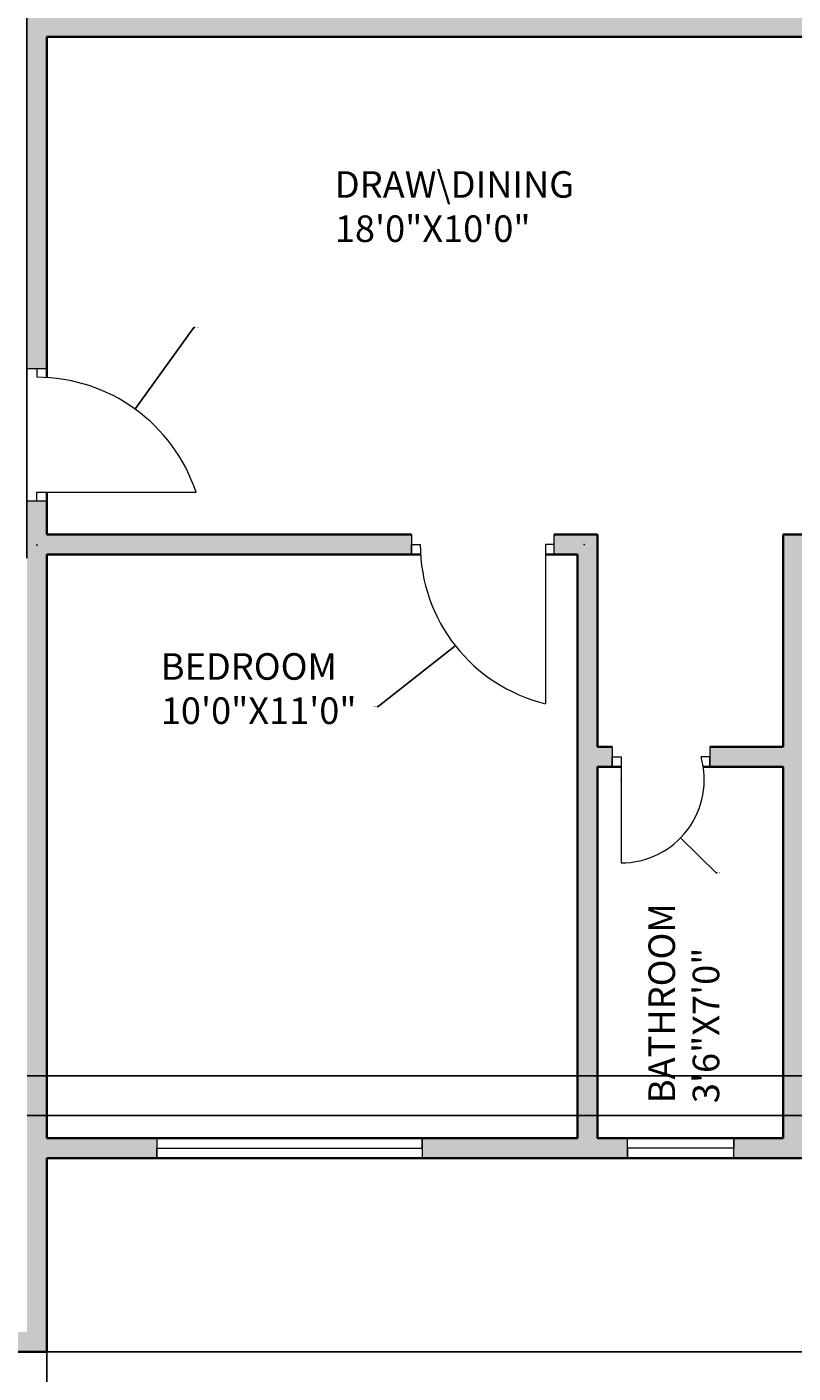
# Model space of a CAD drawing. Units: inches. Extents: x 2314 to 3223, y 1382 to 2735.
# Tile 4 of 14: x 2818 to 2992, y 1560 to 1864. Entities that reach past the tile are written whole.
import ezdxf

# ---------------------------------------------------------------- set-up
doc = ezdxf.new("R2010")
doc.units = ezdxf.units.IN
for name, color, linetype, lineweight in [('A-ANNO-DIMS', 2, 'Continuous', 18), ('A-AREA-IDEN', 7, 'Continuous', 18), ('A-DOOR', 3, 'Continuous', 18), ('A-GLAZ', 4, 'Continuous', 18), ('A-WALL', 7, 'Continuous', 35)]:
    doc.layers.add(name, color=color, linetype=linetype, lineweight=lineweight)
doc.layers.add('A-WALL-PATT', color=251, linetype='Continuous', lineweight=13, true_color=0x636466)
doc.styles.get("Standard").update_dxf_attribs({"font": 'arial.ttf'})
doc.dimstyles.get("Standard").update_dxf_attribs({"dimtxt": 0.18, "dimasz": 0.18, "dimexe": 0.18, "dimexo": 0.0625, "dimgap": 0.09, "dimtad": 0, "dimtih": 1, "dimtoh": 1, "dimdec": 4, "dimzin": 0, "dimdsep": 46, "dimtxsty": 'Standard', "dimcen": 0.09, "dimadec": 0, "dimazin": 0, "dimtfac": 1, "dimtdec": 4, "dimtofl": 0, "dimtmove": 0, "dimatfit": 3, "dimfxl": 1, "dimtolj": 1, "dimtzin": 0, "dimarcsym": 0})

# ---------------------------------------------------------------- blocks, each defined once
blk = doc.blocks.new('WIN-PLAN-24')
for p, q in [((0, 24), (4.5, 24)), ((4.5, 24), (2.25, 24)), ((2.25, 24), (2.25, 0)), ((2.25, 0), (0, 0)), ((0, 0), (4.5, 0))]:
    blk.add_line(p, q)
blk = doc.blocks.new('WIN-PLAN-60')
for p, q in [((0, 4.5), (0, 0)), ((60, 2.25), (60, 4.5)), ((60, 4.5), (60, 0)), ((0, 0), (0, 2.25)), ((0, 2.25), (60, 2.25))]:
    blk.add_line(p, q)
blk = doc.blocks.new('*D29')
at = {"layer": 'A-ANNO-DIMS', "color": 0, "lineweight": -2, "transparency": 16777216}
for p, q in [((2410.39, 1608.32), (2410.39, 1434.13)), ((3125.89, 1608.32), (3125.89, 1434.13)), ((2410.57, 1434.31), (2767.75, 1434.31)), ((3125.71, 1434.31), (2768.54, 1434.31))]:
    blk.add_line(p, q, dxfattribs=at)
at = {"layer": 'A-ANNO-DIMS', "color": 0, "transparency": 16777216}
for points in [[(2410.57, 1434.34), (2410.57, 1434.28), (2410.39, 1434.31)], [(3125.71, 1434.34), (3125.71, 1434.28), (3125.89, 1434.31)]]:
    blk.add_solid(points, dxfattribs=at)
at = {"layer": 'Defpoints', "color": 0, "transparency": 16777216}
for p in [(2410.39, 1608.38), (3125.89, 1608.38), (3125.89, 1434.31)]:
    blk.add_point(p, dxfattribs=at)
at = {"layer": 'A-ANNO-DIMS', "color": 0, "transparency": 16777216, "insert": (2768.14, 1434.31), "char_height": 0.18, "attachment_point": 5}
blk.add_mtext('\\A1;715.5', dxfattribs=at)
blk = doc.blocks.new('*D30')
at = {"layer": 'A-ANNO-DIMS', "color": 0, "lineweight": -2, "transparency": 16777216}
for p, q in [((3125.96, 2381.78), (3172.77, 2381.78)), ((3172.59, 2381.6), (3172.59, 1973.38)), ((3172.59, 1564.8), (3172.59, 1973.02)), ((2822.96, 1564.62), (3172.77, 1564.62))]:
    blk.add_line(p, q, dxfattribs=at)
at = {"layer": 'A-ANNO-DIMS', "color": 0, "transparency": 16777216}
for points in [[(3172.56, 2381.6), (3172.62, 2381.6), (3172.59, 2381.78)], [(3172.56, 1564.8), (3172.62, 1564.8), (3172.59, 1564.62)]]:
    blk.add_solid(points, dxfattribs=at)
at = {"layer": 'Defpoints', "color": 0, "transparency": 16777216}
for p in [(3125.89, 2381.78), (2822.89, 1564.62), (3172.59, 1564.62)]:
    blk.add_point(p, dxfattribs=at)
at = {"layer": 'A-ANNO-DIMS', "color": 0, "transparency": 16777216, "insert": (3172.59, 1973.2), "char_height": 0.18, "attachment_point": 5}
blk.add_mtext('\\A1;817.2', dxfattribs=at)
blk = doc.blocks.new('*D37')
at = {"layer": 'A-ANNO-DIMS', "color": 0, "lineweight": -2, "transparency": 16777216}
for p, q in [((2717.89, 1564.56), (2717.89, 1434.13)), ((2822.89, 1564.56), (2822.89, 1434.13)), ((2718.07, 1434.31), (2770.11, 1434.31)), ((2822.71, 1434.31), (2770.67, 1434.31))]:
    blk.add_line(p, q, dxfattribs=at)
at = {"layer": 'A-ANNO-DIMS', "color": 0, "transparency": 16777216}
for points in [[(2718.07, 1434.34), (2718.07, 1434.28), (2717.89, 1434.31)], [(2822.71, 1434.34), (2822.71, 1434.28), (2822.89, 1434.31)]]:
    blk.add_solid(points, dxfattribs=at)
at = {"layer": 'Defpoints', "color": 0, "transparency": 16777216}
for p in [(2717.89, 1564.62), (2822.89, 1564.62), (2822.89, 1434.31)]:
    blk.add_point(p, dxfattribs=at)
at = {"layer": 'A-ANNO-DIMS', "color": 0, "transparency": 16777216, "insert": (2770.39, 1434.31), "char_height": 0.18, "attachment_point": 5}
blk.add_mtext('\\A1;105', dxfattribs=at)
blk = doc.blocks.new('*D38')
at = {"layer": 'A-ANNO-DIMS', "color": 0, "lineweight": -2, "transparency": 16777216}
for p, q in [((2818.46, 1627), (3172.77, 1627)), ((3172.59, 1626.82), (3172.59, 1622.68)), ((3172.59, 1618.18), (3172.59, 1622.32)), ((2818.46, 1618), (3172.77, 1618))]:
    blk.add_line(p, q, dxfattribs=at)
at = {"layer": 'A-ANNO-DIMS', "color": 0, "transparency": 16777216}
for points in [[(3172.56, 1626.82), (3172.62, 1626.82), (3172.59, 1627)], [(3172.56, 1618.18), (3172.62, 1618.18), (3172.59, 1618)]]:
    blk.add_solid(points, dxfattribs=at)
at = {"layer": 'Defpoints', "color": 0, "transparency": 16777216}
for p in [(2818.39, 1627), (3172.59, 1627), (2818.39, 1618)]:
    blk.add_point(p, dxfattribs=at)
at = {"layer": 'A-ANNO-DIMS', "color": 0, "transparency": 16777216, "insert": (3172.59, 1622.5), "char_height": 0.18, "attachment_point": 5}
blk.add_mtext('\\A1;9', dxfattribs=at)
blk = doc.blocks.new('*D39')
at = {"layer": 'A-ANNO-DIMS', "color": 0, "lineweight": -2, "transparency": 16777216}
for p, q in [((2770.39, 1744.06), (2770.39, 2428.66)), ((2818.39, 1744.06), (2818.39, 2428.66)), ((2770.57, 2428.48), (2794.17, 2428.48)), ((2818.21, 2428.48), (2794.62, 2428.48))]:
    blk.add_line(p, q, dxfattribs=at)
at = {"layer": 'A-ANNO-DIMS', "color": 0, "transparency": 16777216}
for points in [[(2770.57, 2428.51), (2770.57, 2428.45), (2770.39, 2428.48)], [(2818.21, 2428.51), (2818.21, 2428.45), (2818.39, 2428.48)]]:
    blk.add_solid(points, dxfattribs=at)
at = {"layer": 'Defpoints', "color": 0, "transparency": 16777216}
for p in [(2818.39, 2428.48), (2770.39, 1744), (2818.39, 1744)]:
    blk.add_point(p, dxfattribs=at)
at = {"layer": 'A-ANNO-DIMS', "color": 0, "transparency": 16777216, "insert": (2794.39, 2428.48), "char_height": 0.18, "attachment_point": 5}
blk.add_mtext('\\A1;48', dxfattribs=at)
blk = doc.blocks.new('*D60')
at = {"layer": 'A-ANNO-DIMS', "color": 0, "lineweight": -2, "transparency": 16777216}
for p, q in [((2856.17, 1796.19), (2842.95, 1777.89)), ((2856.35, 1796.19), (2856.17, 1796.19)), ((2820.55, 1747), (2820.73, 1747)), ((2820.64, 1746.91), (2820.64, 1747.09))]:
    blk.add_line(p, q, dxfattribs=at)
at = {"layer": 'A-ANNO-DIMS', "color": 0, "transparency": 16777216}
blk.add_solid([(2842.93, 1777.91), (2842.98, 1777.87), (2842.85, 1777.74)], dxfattribs=at)
at = {"layer": 'Defpoints', "color": 0, "transparency": 16777216}
for p in [(2842.85, 1777.74), (2820.64, 1747)]:
    blk.add_point(p, dxfattribs=at)
at = {"layer": 'A-ANNO-DIMS', "color": 0, "transparency": 16777216, "insert": (2856.83, 1796.19), "char_height": 0.18, "attachment_point": 5}
blk.add_mtext('\\A1;R37.92', dxfattribs=at)
blk = doc.blocks.new('*D62')
at = {"layer": 'A-ANNO-DIMS', "color": 0, "lineweight": -2, "transparency": 16777216}
for p, q in [((2944.31, 1747.13), (2944.49, 1747.13)), ((2944.4, 1747.04), (2944.4, 1747.22)), ((2897.8, 1710.5), (2915.13, 1724.13)), ((2897.62, 1710.5), (2897.8, 1710.5))]:
    blk.add_line(p, q, dxfattribs=at)
at = {"layer": 'A-ANNO-DIMS', "color": 0, "transparency": 16777216}
blk.add_solid([(2915.11, 1724.15), (2915.15, 1724.1), (2915.27, 1724.24)], dxfattribs=at)
at = {"layer": 'Defpoints', "color": 0, "transparency": 16777216}
for p in [(2944.4, 1747.13), (2915.27, 1724.24)]:
    blk.add_point(p, dxfattribs=at)
at = {"layer": 'A-ANNO-DIMS', "color": 0, "transparency": 16777216, "insert": (2897.14, 1710.5), "char_height": 0.18, "attachment_point": 5}
blk.add_mtext('\\A1;R37.05', dxfattribs=at)
blk = doc.blocks.new('*D94')
at = {"layer": 'A-ANNO-DIMS', "color": 0, "lineweight": -2, "transparency": 16777216}
for p, q in [((2952.67, 1693.93), (2952.85, 1693.93)), ((2952.76, 1693.84), (2952.76, 1694.02)), ((2974.26, 1672.9), (2966.32, 1680.66)), ((2974.44, 1672.9), (2974.26, 1672.9))]:
    blk.add_line(p, q, dxfattribs=at)
at = {"layer": 'A-ANNO-DIMS', "color": 0, "transparency": 16777216}
blk.add_solid([(2966.35, 1680.68), (2966.3, 1680.64), (2966.2, 1680.79)], dxfattribs=at)
at = {"layer": 'Defpoints', "color": 0, "transparency": 16777216}
for p in [(2952.76, 1693.93), (2966.2, 1680.79)]:
    blk.add_point(p, dxfattribs=at)
at = {"layer": 'A-ANNO-DIMS', "color": 0, "transparency": 16777216, "insert": (2974.85, 1672.9), "char_height": 0.18, "attachment_point": 5}
blk.add_mtext('\\A1;R18.8', dxfattribs=at)

msp = doc.modelspace()

# ---------------------------------------------------------------- hatches: boundary and pattern name
at = {"layer": 'A-WALL-PATT'}
h = msp.add_hatch(color=256, dxfattribs=at)
h.dxf.hatch_style = 1
h.paths.add_polyline_path([(2443.3302, 2379.5332), (2443.3302, 2381.7832), (2410.3927, 2381.7832), (2410.3927, 2336.7008), (2414.8927, 2336.7008), (2414.8927, 2377.2832), (2443.3302, 2377.2832)])
h.paths.add_polyline_path([(2561.3645, 2379.5332), (2561.3645, 2381.7832), (2503.3302, 2381.7832), (2503.3302, 2377.2832), (2546.8927, 2377.2832), (2546.8927, 2245.2832), (2541.8787, 2245.2832), (2541.8787, 2240.7832), (2551.3927, 2240.7832), (2551.3927, 2377.2832), (2561.3645, 2377.2832)])
h.paths.add_polyline_path([(2656.0607, 2381.7832), (2597.3645, 2381.7832), (2597.3645, 2377.2832), (2617.3927, 2377.2832), (2617.3927, 2257.2832), (2584.2532, 2257.2832), (2584.2532, 2252.7832), (2625.8528, 2252.7832), (2625.8528, 2255.0332), (2625.8528, 2257.2832), (2621.8927, 2257.2832), (2621.8927, 2377.2832), (2656.0607, 2377.2832), (2656.0607, 2379.5332)])
h.paths.add_polyline_path([(2807.3418, 2381.7832), (2716.0607, 2381.7832), (2716.0607, 2377.2832), (2765.8927, 2377.2832), (2765.8927, 2257.2832), (2661.6935, 2257.2832), (2661.6935, 2252.7832), (2765.8927, 2252.7832), (2765.8927, 2146.2832), (2760.9259, 2146.2832), (2760.9259, 2141.8832), (2775.7119, 2141.8832), (2775.7119, 2146.2832), (2770.3927, 2146.2832), (2770.3927, 2252.7832), (2877.684, 2252.7832), (2877.684, 2255.0332), (2877.684, 2257.2832), (2770.3927, 2257.2832), (2770.3927, 2377.2832), (2807.3418, 2377.2832), (2807.3418, 2379.5332)])
h.paths.add_polyline_path([(2937.2118, 2381.7832), (2867.3418, 2381.7832), (2867.3418, 2377.2832), (2914.3927, 2377.2832), (2914.3927, 2257.2832), (2908.4124, 2257.2832), (2908.4124, 2252.7832), (2960.6432, 2252.7832), (2960.6432, 2255.0332), (2960.6432, 2257.2832), (2918.8927, 2257.2832), (2918.8927, 2377.2832), (2937.2118, 2377.2832)])
h.paths.add_polyline_path([(3022.1601, 2381.7832), (2973.2118, 2381.7832), (2973.2118, 2379.5332), (2973.2118, 2377.2832), (2984.8927, 2377.2832), (2984.8927, 2257.2832), (2980.0601, 2257.2832), (2980.0601, 2252.7832), (2984.8927, 2252.7832), (2984.8927, 2240.7832), (2995.668, 2240.7832), (2995.668, 2243.0332), (2995.668, 2245.2832), (2989.3927, 2245.2832), (2989.3927, 2377.2832), (3022.1601, 2377.2832), (3022.1601, 2379.5332)])
h.paths.add_polyline_path([(3125.8927, 2381.7832), (3082.1601, 2381.7832), (3082.1601, 2377.2832), (3121.3927, 2377.2832), (3121.3927, 2334.7388), (3125.8927, 2334.7388)])
h.paths.add_polyline_path([(3125.8927, 2274.7388), (3121.3927, 2274.7388), (3121.3927, 2245.2832), (3066.4832, 2245.2832), (3066.4832, 2240.7832), (3121.3927, 2240.7832), (3121.3927, 2232.1868), (3125.8927, 2232.1868)])
h.paths.add_polyline_path([(3125.8927, 2208.1868), (3121.3927, 2208.1868), (3121.3927, 2198.7832), (3037.3927, 2198.7832), (3037.3927, 2240.7832), (3041.2694, 2240.7832), (3041.2694, 2243.0332), (3041.2694, 2245.2832), (3026.8205, 2245.2832), (3026.8205, 2240.7832), (3032.8927, 2240.7832), (3032.8927, 2190.4022), (3037.3927, 2190.4022), (3037.3927, 2194.2832), (3121.3927, 2194.2832), (3121.3927, 2182.1835), (3125.8927, 2182.1835)])
h.paths.add_polyline_path([(3125.8927, 2158.1835), (3121.3927, 2158.1835), (3121.3927, 2146.2832), (3037.3927, 2146.2832), (3037.3927, 2169.3726), (3035.1427, 2169.3726), (3032.8927, 2169.3726), (3032.8927, 2146.2832), (2812.7301, 2146.2832), (2812.7301, 2144.0832), (2812.7301, 2141.8832), (2818.3927, 2141.8832), (2818.3927, 1970.1316), (2822.8927, 1970.1316), (2822.8927, 1978.8832), (2903.9846, 1978.8832), (2903.9846, 1981.1332), (2903.9846, 1983.3832), (2822.8927, 1983.3832), (2822.8927, 2115.3832), (2851.7162, 2115.3832), (2851.7162, 2117.6332), (2851.7162, 2119.8832), (2822.8927, 2119.8832), (2822.8927, 2141.8832), (3125.8927, 2141.8832)])
h.paths.add_polyline_path([(3125.8927, 2119.8832), (3081.193, 2119.8832), (3081.193, 2115.3832), (3121.3927, 2115.3832), (3121.3927, 2071.8188), (3125.8927, 2071.8188)], flags=17)
h.paths.add_polyline_path([(2989.3927, 2115.3832), (3021.193, 2115.3832), (3021.193, 2117.6332), (3021.193, 2119.8832), (2979.123, 2119.8832), (2979.123, 2115.3832), (2984.8927, 2115.3832), (2984.8927, 2019.3832), (2981.9225, 2019.3832), (2981.9225, 2014.8832), (2984.8927, 2014.8832), (2984.8927, 1983.3832), (2984.8927, 1978.8832), (2989.3927, 1978.8832), (2989.3927, 1983.3832)], flags=17)
h.paths.add_polyline_path([(2947.3927, 2115.3832), (2955.123, 2115.3832), (2955.123, 2117.6332), (2955.123, 2119.8832), (2911.7162, 2119.8832), (2911.7162, 2115.3832), (2942.8927, 2115.3832), (2942.8927, 1983.3832), (2936.7017, 1983.3832), (2936.7017, 1978.8832), (2947.3927, 1978.8832), (2947.3927, 1983.3832), (2947.3927, 2014.8832), (2960.7167, 2014.8832), (2960.7167, 2017.1332), (2960.7167, 2019.3832), (2947.3927, 2019.3832)], flags=17)
h.paths.add_polyline_path([(3037.3927, 1978.8832), (3041.8276, 1978.8832), (3041.8276, 1981.1332), (3041.8276, 1983.3832), (3025.477, 1983.3832), (3025.477, 1978.8832), (3032.8927, 1978.8832), (3032.8927, 1927.1259), (3035.1427, 1927.1259), (3037.3927, 1927.1259)])
h.paths.add_polyline_path([(3125.8927, 2011.8188), (3123.6427, 2011.8188), (3121.3927, 2011.8188), (3121.3927, 1983.3832), (3065, 1983.3832), (3065, 1978.8832), (3121.3927, 1978.8832), (3121.3927, 1970.5932), (3125.8927, 1970.5932)], flags=17)
h.paths.add_polyline_path([(2994.2341, 1983.3832), (2989.3927, 1983.3832), (2989.3927, 1978.8832), (2994.2341, 1978.8832), (2994.2341, 1981.1332)], flags=16)
h.paths.add_polyline_path([(3125.8927, 1946.5932), (3121.3927, 1946.5932), (3121.3927, 1936.8832), (3037.3927, 1936.8832), (3037.3927, 1932.3832), (3121.3927, 1932.3832), (3121.3927, 1919.825), (3125.8927, 1919.825)])
h.paths.add_polyline_path([(3125.8927, 1883.825), (3121.3927, 1883.825), (3121.3927, 1866.3832), (3037.3927, 1866.3832), (3037.3927, 1899.0954), (3035.1427, 1899.0954), (3032.8927, 1899.0954), (3032.8927, 1866.3832), (2822.8927, 1866.3832), (2822.8927, 1938.7212), (2820.6427, 1938.7212), (2818.3927, 1938.7212), (2818.3927, 1786.9239), (2822.8927, 1786.9239), (2822.8927, 1861.8832), (3032.8927, 1861.8832), (3032.8927, 1825.1023), (3037.3927, 1825.1023), (3037.3927, 1861.8832), (3121.3927, 1861.8832), (3121.3927, 1844.6765), (3125.8927, 1844.6765)])
h.paths.add_polyline_path([(3125.8927, 1808.6765), (3121.3927, 1808.6765), (3121.3927, 1795.8832), (3037.3927, 1795.8832), (3037.3927, 1799.4755), (3032.8927, 1799.4755), (3032.8927, 1749.3832), (3026.5034, 1749.3832), (3026.5034, 1744.8832), (3032.8927, 1744.8832), (3034.9255, 1744.8832), (3043.1326, 1744.8832), (3043.1326, 1747.1332), (3043.1326, 1749.3832), (3037.3927, 1749.3832), (3037.3927, 1791.3832), (3121.3927, 1791.3832), (3121.3927, 1783.3103), (3125.8927, 1783.3103)])
h.paths.add_polyline_path([(3125.8927, 1759.3103), (3121.3927, 1759.3103), (3121.3927, 1749.3832), (3065.1845, 1749.3832), (3065.1845, 1744.8832), (3121.3927, 1744.8832), (3121.3927, 1709.3573), (3125.8927, 1709.3573)])
h.paths.add_polyline_path([(3125.8927, 1649.3573), (3121.3927, 1649.3573), (3121.3927, 1612.8832), (3095.116, 1612.8832), (3095.116, 1608.3832), (3125.8927, 1608.3832)])
h.paths.add_polyline_path([(3035.116, 1612.8832), (2993.8927, 1612.8832), (2993.8927, 1744.8832), (2998.7409, 1744.8832), (2998.7409, 1749.3832), (2989.3927, 1749.3832), (2989.3927, 1744.8832), (2989.3927, 1701.3832), (2972.8226, 1701.3832), (2972.8226, 1696.8832), (2989.3927, 1696.8832), (2989.3927, 1612.8832), (2978.2225, 1612.8832), (2978.2225, 1608.3832), (3035.116, 1608.3832), (3035.116, 1610.6332)])
h.paths.add_polyline_path([(2947.3927, 1696.8832), (2950.7566, 1696.8832), (2950.7566, 1699.1332), (2950.7566, 1701.3832), (2947.3927, 1701.3832), (2947.3927, 1744.8832), (2947.3927, 1749.3832), (2937.649, 1749.3832), (2937.649, 1744.8832), (2942.8927, 1744.8832), (2942.8927, 1612.8832), (2907.783, 1612.8832), (2907.783, 1608.3832), (2954.2225, 1608.3832), (2954.2225, 1610.6332), (2954.2225, 1612.8832), (2947.3927, 1612.8832)])
h.paths.add_polyline_path([(2822.8927, 1744.8832), (2905.3491, 1744.8832), (2905.3491, 1747.1332), (2905.3491, 1749.3832), (2822.8927, 1749.3832), (2822.8927, 1756.9185), (2818.3927, 1756.9185), (2818.3927, 1612.8832), (2818.3927, 1569.1205), (2722.3927, 1569.1205), (2722.3927, 1612.8832), (2722.3927, 1756.9185), (2717.8927, 1756.9185), (2717.8927, 1750.0143), (2633.6297, 1750.0143), (2633.6437, 1745.2665), (2717.8927, 1745.5143), (2717.8927, 1612.8832), (2689.8467, 1612.8832), (2689.8467, 1608.3832), (2717.8927, 1608.3832), (2717.8927, 1564.6205), (2722.3927, 1564.6205), (2822.8927, 1564.6205), (2822.8927, 1569.1205), (2822.8927, 1608.3832), (2847.783, 1608.3832), (2847.783, 1610.6332), (2847.783, 1612.8832), (2822.8927, 1612.8832)])
h.paths.add_polyline_path([(2629.8467, 1612.8832), (2597.8927, 1612.8832), (2597.8927, 1744.8832), (2597.8927, 1745.1613), (2601.5887, 1745.1721), (2601.5816, 1747.5932), (2601.5745, 1750.0143), (2593.3927, 1750.0143), (2593.3927, 1744.8832), (2593.3927, 1713.3832), (2589.7588, 1713.3832), (2589.7588, 1708.8832), (2593.3927, 1708.8832), (2593.3927, 1612.8832), (2582.3793, 1612.8832), (2582.3793, 1608.3832), (2629.8467, 1608.3832), (2629.8467, 1610.6332)])
h.paths.add_polyline_path([(2551.3927, 1708.8832), (2567.6776, 1708.8832), (2567.6776, 1711.1332), (2567.6776, 1713.3832), (2551.3927, 1713.3832), (2551.3927, 1744.8832), (2551.3927, 1750.0143), (2543.5657, 1750.0143), (2543.5657, 1747.5079), (2543.5657, 1745.0014), (2546.8927, 1745.0112), (2546.8927, 1744.8832), (2546.8927, 1612.8832), (2502.9339, 1612.8832), (2502.9339, 1608.3832), (2558.3793, 1608.3832), (2558.3793, 1610.6332), (2558.3793, 1612.8832), (2551.3927, 1612.8832)])
h.paths.add_polyline_path([(2414.8927, 1656.2547), (2410.3927, 1656.2547), (2410.3927, 1608.3832), (2442.9339, 1608.3832), (2442.9339, 1610.6332), (2442.9339, 1612.8832), (2414.8927, 1612.8832)])
h.paths.add_polyline_path([(2414.8927, 1744.8832), (2468.8906, 1744.8832), (2468.8906, 1747.1332), (2468.8906, 1749.3832), (2414.8927, 1749.3832), (2414.8927, 1757.7622), (2410.3927, 1757.7622), (2410.3927, 1716.2547), (2414.8927, 1716.2547)])
h.paths.add_polyline_path([(2414.8927, 1791.3832), (2498.8927, 1791.3832), (2498.8927, 1749.3832), (2492.9799, 1749.3832), (2492.9799, 1744.8832), (2498.8927, 1744.8832), (2503.3927, 1744.8832), (2508.0135, 1744.8968), (2508.0059, 1747.4556), (2507.9984, 1750.0143), (2503.3927, 1750.0143), (2503.3927, 1802.6362), (2501.1427, 1802.6362), (2498.8927, 1802.6362), (2498.8927, 1795.8832), (2414.8927, 1795.8832), (2414.8927, 1808.0943), (2410.3927, 1808.0943), (2410.3927, 1781.7622), (2414.8927, 1781.7622)])
h.paths.add_polyline_path([(2722.3927, 1937.589), (2720.1427, 1937.589), (2717.8927, 1937.589), (2717.8927, 1866.3832), (2503.3927, 1866.3832), (2503.3927, 1896.3484), (2498.8927, 1896.3484), (2498.8927, 1866.3832), (2414.8927, 1866.3832), (2414.8927, 1882.1496), (2410.3927, 1882.1496), (2410.3927, 1844.0943), (2414.8927, 1844.0943), (2414.8927, 1861.8832), (2498.8927, 1861.8832), (2498.8927, 1831.4783), (2501.1427, 1831.4783), (2503.3927, 1831.4783), (2503.3927, 1861.8832), (2717.8927, 1861.8832), (2717.8927, 1786.9239), (2722.3927, 1786.9239)])
h.paths.add_polyline_path([(2414.8927, 1932.3832), (2498.8927, 1932.3832), (2498.8927, 1924.7883), (2503.3927, 1924.7883), (2503.3927, 1978.8832), (2505.8599, 1978.8832), (2505.8599, 1981.1332), (2505.8599, 1983.3832), (2493.3697, 1983.3832), (2493.3697, 1978.8832), (2498.8927, 1978.8832), (2498.8927, 1936.8832), (2414.8927, 1936.8832), (2414.8927, 1943.2834), (2410.3927, 1943.2834), (2410.3927, 1918.1496), (2414.8927, 1918.1496)])
h.paths.add_polyline_path([(2414.8927, 2020.3133), (2412.6427, 2020.3133), (2410.3927, 2020.3133), (2410.3927, 1967.2834), (2414.8927, 1967.2834), (2414.8927, 1978.8832), (2468.8513, 1978.8832), (2468.8513, 1981.1332), (2468.8513, 1983.3832), (2414.8927, 1983.3832)])
h.paths.add_polyline_path([(2414.8927, 2115.3832), (2453.004, 2115.3832), (2453.004, 2117.6332), (2453.004, 2119.8832), (2410.3927, 2119.8832), (2410.3927, 2080.3133), (2414.8927, 2080.3133)], flags=17)
h.paths.add_polyline_path([(2559.0969, 2117.6332), (2559.0969, 2119.8832), (2513.004, 2119.8832), (2513.004, 2115.3832), (2546.8927, 2115.3832), (2546.8927, 1983.3832), (2542.7531, 1983.3832), (2542.7531, 1978.8832), (2551.3927, 1978.8832), (2551.3927, 2014.8832), (2570.3098, 2014.8832), (2570.3098, 2017.1332), (2570.3098, 2019.3832), (2551.3927, 2019.3832), (2551.3927, 2115.3832), (2559.0969, 2115.3832)], flags=17)
h.paths.add_polyline_path([(2628.5073, 2117.6332), (2628.5073, 2119.8832), (2583.0969, 2119.8832), (2583.0969, 2115.3832), (2593.3927, 2115.3832), (2593.3927, 2019.3832), (2590.2108, 2019.3832), (2590.2108, 2014.8832), (2593.3927, 2014.8832), (2593.3927, 1978.8832), (2601.5907, 1978.8832), (2601.5907, 1981.1332), (2601.5907, 1983.3832), (2597.8927, 1983.3832), (2597.8927, 2115.3832), (2628.5073, 2115.3832)], flags=17)
h.paths.add_polyline_path([(2722.3927, 2141.8832), (2726.9871, 2141.8832), (2726.9871, 2144.2705), (2726.9871, 2146.2832), (2503.3927, 2146.2832), (2503.3927, 2168.2161), (2501.1427, 2168.2161), (2498.8927, 2168.2161), (2498.8927, 2146.2832), (2414.8927, 2146.2832), (2414.8927, 2156.5041), (2410.3927, 2156.5041), (2410.3927, 2141.8832), (2717.8927, 2141.8832), (2717.8927, 2119.8832), (2688.5073, 2119.8832), (2688.5073, 2115.3832), (2717.8927, 2115.3832), (2717.8927, 1983.3832), (2633.2454, 1983.3832), (2633.2454, 1978.8832), (2717.8927, 1978.8832), (2717.8927, 1970.1316), (2720.1427, 1970.1316), (2722.3927, 1970.1316)])
h.paths.add_polyline_path([(2557.3704, 1462.9278), (2940.0934, 1462.9278), (2940.0934, 1512.3848), (2557.3704, 1512.3848)], flags=9)
h.paths.add_polyline_path([(2846.2527, 1703.1384), (2892.8612, 1703.1384), (2892.8612, 1725.5272), (2846.2527, 1725.5272)], flags=25)
h.paths.add_polyline_path([(2885.6102, 1812.1147), (2946.1505, 1812.1147), (2946.1505, 1834.5035), (2885.6102, 1834.5035)], flags=25)
h.paths.add_polyline_path([(2885.6102, 1884.183), (2946.1505, 1884.183), (2946.1505, 1906.5718), (2885.6102, 1906.5718)], flags=25)
h.paths.add_polyline_path([(3066.365, 1705.5431), (3112.9735, 1705.5431), (3112.9735, 1727.9319), (3066.365, 1727.9319)], flags=9)
h.paths.add_polyline_path([(3061.8255, 1887.7513), (3101.6154, 1887.7513), (3101.6154, 1910.1401), (3061.8255, 1910.1401)], flags=25)
h.paths.add_polyline_path([(3063.3679, 1816.2121), (3103.1578, 1816.2121), (3103.1578, 1838.6009), (3063.3679, 1838.6009)], flags=25)
h.paths.add_polyline_path([(3053.3743, 1768.416), (3107.1329, 1768.416), (3107.1329, 1790.8048), (3053.3743, 1790.8048)], flags=25)
h.paths.add_polyline_path([(3061.6068, 1943.822), (3115.3653, 1943.822), (3115.3653, 1966.2109), (3061.6068, 1966.2109)], flags=9)
h.paths.add_polyline_path([(2745.0978, 1763.6604), (2797.9354, 1763.6604), (2797.9354, 1776.0247), (2745.0978, 1776.0247)], flags=9)
h.paths.add_polyline_path([(2574.2135, 1819.2586), (2634.7538, 1819.2586), (2634.7538, 1841.6474), (2574.2135, 1841.6474)], flags=25)
h.paths.add_polyline_path([(2574.2135, 1891.3269), (2634.7538, 1891.3269), (2634.7538, 1913.7157), (2574.2135, 1913.7157)], flags=25)
h.paths.add_polyline_path([(2638.4466, 1702.43), (2685.0551, 1702.43), (2685.0551, 1724.8188), (2638.4466, 1724.8188)], flags=25)
h.paths.add_polyline_path([(2435.9715, 1697.1215), (2482.5799, 1697.1215), (2482.5799, 1719.5103), (2435.9715, 1719.5103)], flags=9)
h.paths.add_polyline_path([(2431.2046, 1893.7833), (2470.9945, 1893.7833), (2470.9945, 1916.1721), (2431.2046, 1916.1721)], flags=25)
h.paths.add_polyline_path([(2439.8144, 1817.2116), (2479.6043, 1817.2116), (2479.6043, 1839.6004), (2439.8144, 1839.6004)], flags=25)
h.paths.add_polyline_path([(2441.2607, 1753.0942), (2495.0192, 1753.0942), (2495.0192, 1775.483), (2441.2607, 1775.483)], flags=25)
h.paths.add_polyline_path([(2421.216, 1945.3109), (2474.9746, 1945.3109), (2474.9746, 1967.6997), (2421.216, 1967.6997)], flags=25)
h.paths.add_polyline_path([(2585.4464, 1627.5703), (2585.4464, 1679), (2563.0576, 1679), (2563.0576, 1627.5703)], flags=9)
h.paths.add_polyline_path([(2978.3497, 1618.7039), (2978.3497, 1670.1337), (2955.9609, 1670.1337), (2955.9609, 1618.7039)], flags=9)
h.paths.add_polyline_path([(2975.9502, 2041.7828), (2975.9502, 2093.2125), (2953.5614, 2093.2125), (2953.5614, 2041.7828)], flags=25)
h.paths.add_polyline_path([(2835.6537, 1989.2068), (2882.2621, 1989.2068), (2882.2621, 2011.5956), (2835.6537, 2011.5956)], flags=25)
h.paths.add_polyline_path([(2649.3769, 1997.5659), (2695.9853, 1997.5659), (2695.9853, 2019.9547), (2649.3769, 2019.9547)], flags=25)
h.paths.add_polyline_path([(2579.9087, 2040.3429), (2579.9087, 2091.7726), (2557.5198, 2091.7726), (2557.5198, 2040.3429)], flags=25)
h.paths.add_polyline_path([(2783.2404, 1883.1956), (2783.2404, 2067.1369), (2764.694, 2067.1369), (2764.694, 1883.1956)], flags=9)
h.paths.add_polyline_path([(3055.8435, 1993.5571), (3102.4519, 1993.5571), (3102.4519, 2015.9459), (3055.8435, 2015.9459)], flags=25)
h.paths.add_polyline_path([(2423.6009, 1984.6082), (2470.2094, 1984.6082), (2470.2094, 2006.997), (2423.6009, 2006.997)], flags=25)
h.paths.add_polyline_path([(2973.4115, 2123.1668), (3013.1319, 2123.1668), (3013.1319, 2135.531), (2973.4115, 2135.531)], flags=25)
h.paths.add_polyline_path([(2534.3846, 2124.6231), (2574.105, 2124.6231), (2574.105, 2136.9874), (2534.3846, 2136.9874)], flags=25)
h.paths.add_polyline_path([(2829.1368, 2188.1931), (2889.411, 2188.1931), (2889.411, 2210.5819), (2829.1368, 2210.5819)], flags=9)
h.paths.add_polyline_path([(2633.2547, 2185.0437), (2693.5289, 2185.0437), (2693.5289, 2207.4325), (2633.2547, 2207.4325)], flags=9)
h.paths.add_polyline_path([(2445.1812, 2167.0395), (2496.611, 2167.0395), (2496.611, 2189.4284), (2445.1812, 2189.4284)], flags=9)
h.paths.add_polyline_path([(2429.1678, 2194.5482), (2480.5975, 2194.5482), (2480.5975, 2216.937), (2429.1678, 2216.937)], flags=9)
h.paths.add_polyline_path([(3060.1138, 2158.1056), (3111.5436, 2158.1056), (3111.5436, 2180.4944), (3060.1138, 2180.4944)], flags=9)
h.paths.add_polyline_path([(3055.6824, 2201.2631), (3107.1122, 2201.2631), (3107.1122, 2223.652), (3055.6824, 2223.652)], flags=25)
h.paths.add_polyline_path([(3044.3482, 2257.7345), (3090.9567, 2257.7345), (3090.9567, 2280.1233), (3044.3482, 2280.1233)], flags=9)
h.paths.add_polyline_path([(2942.5437, 2306.9625), (2982.3336, 2306.9625), (2982.3336, 2329.3513), (2942.5437, 2329.3513)], flags=9)
h.paths.add_polyline_path([(2799.5865, 2259.1663), (2846.195, 2259.1663), (2846.195, 2281.5551), (2799.5865, 2281.5551)], flags=25)
h.paths.add_polyline_path([(2670.4998, 2261.1493), (2717.1082, 2261.1493), (2717.1082, 2283.5381), (2670.4998, 2283.5381)], flags=25)
h.paths.add_polyline_path([(2553.0333, 2302.7735), (2592.8232, 2302.7735), (2592.8232, 2325.1624), (2553.0333, 2325.1624)], flags=9)
h.paths.add_polyline_path([(2432.0288, 2268.6489), (2478.6372, 2268.6489), (2478.6372, 2291.0377), (2432.0288, 2291.0377)], flags=9)
h = msp.add_hatch(color=256, dxfattribs=at)
h.dxf.hatch_style = 1
h.paths.add_polyline_path([(2503.3927, 2240.7832), (2507.7952, 2240.7832), (2507.7952, 2245.2832), (2496.4262, 2245.2832), (2496.4262, 2243.0332), (2496.4262, 2240.7832), (2498.8927, 2240.7832), (2498.8927, 2198.7832), (2414.8927, 2198.7832), (2414.8927, 2206.5718), (2410.3927, 2206.5718), (2410.3927, 2180.5041), (2412.6427, 2180.5041), (2414.8927, 2180.5041), (2414.8927, 2194.2832), (2498.8927, 2194.2832), (2498.8927, 2191.0069), (2503.3927, 2191.0069)])
h.paths.add_polyline_path([(2414.8927, 2276.7008), (2410.3927, 2276.7008), (2410.3927, 2230.5718), (2414.8927, 2230.5718), (2414.8927, 2240.7832), (2474.2564, 2240.7832), (2474.2564, 2243.0332), (2474.2564, 2245.2832), (2414.8927, 2245.2832)])
h.paths.add_polyline_path([(2557.3704, 1462.9278), (2940.0934, 1462.9278), (2940.0934, 1512.3848), (2557.3704, 1512.3848)], flags=9)
h.paths.add_polyline_path([(2846.2527, 1703.1384), (2892.8612, 1703.1384), (2892.8612, 1725.5272), (2846.2527, 1725.5272)], flags=9)
h.paths.add_polyline_path([(2885.6102, 1812.1147), (2946.1505, 1812.1147), (2946.1505, 1834.5035), (2885.6102, 1834.5035)], flags=9)
h.paths.add_polyline_path([(2885.6102, 1884.183), (2946.1505, 1884.183), (2946.1505, 1906.5718), (2885.6102, 1906.5718)], flags=9)
h.paths.add_polyline_path([(3066.365, 1705.5431), (3112.9735, 1705.5431), (3112.9735, 1727.9319), (3066.365, 1727.9319)], flags=9)
h.paths.add_polyline_path([(3061.8255, 1887.7513), (3101.6154, 1887.7513), (3101.6154, 1910.1401), (3061.8255, 1910.1401)], flags=9)
h.paths.add_polyline_path([(3063.3679, 1816.2121), (3103.1578, 1816.2121), (3103.1578, 1838.6009), (3063.3679, 1838.6009)], flags=9)
h.paths.add_polyline_path([(3053.3743, 1768.416), (3107.1329, 1768.416), (3107.1329, 1790.8048), (3053.3743, 1790.8048)], flags=9)
h.paths.add_polyline_path([(3061.6068, 1943.822), (3115.3653, 1943.822), (3115.3653, 1966.2109), (3061.6068, 1966.2109)], flags=9)
h.paths.add_polyline_path([(2745.0978, 1763.6604), (2797.9354, 1763.6604), (2797.9354, 1776.0247), (2745.0978, 1776.0247)], flags=9)
h.paths.add_polyline_path([(2574.2135, 1819.2586), (2634.7538, 1819.2586), (2634.7538, 1841.6474), (2574.2135, 1841.6474)], flags=9)
h.paths.add_polyline_path([(2574.2135, 1891.3269), (2634.7538, 1891.3269), (2634.7538, 1913.7157), (2574.2135, 1913.7157)], flags=9)
h.paths.add_polyline_path([(2638.4466, 1702.43), (2685.0551, 1702.43), (2685.0551, 1724.8188), (2638.4466, 1724.8188)], flags=9)
h.paths.add_polyline_path([(2435.9715, 1697.1215), (2482.5799, 1697.1215), (2482.5799, 1719.5103), (2435.9715, 1719.5103)], flags=9)
h.paths.add_polyline_path([(2431.2046, 1893.7833), (2470.9945, 1893.7833), (2470.9945, 1916.1721), (2431.2046, 1916.1721)], flags=9)
h.paths.add_polyline_path([(2439.8144, 1817.2116), (2479.6043, 1817.2116), (2479.6043, 1839.6004), (2439.8144, 1839.6004)], flags=9)
h.paths.add_polyline_path([(2441.2607, 1753.0942), (2495.0192, 1753.0942), (2495.0192, 1775.483), (2441.2607, 1775.483)], flags=9)
h.paths.add_polyline_path([(2421.216, 1945.3109), (2474.9746, 1945.3109), (2474.9746, 1967.6997), (2421.216, 1967.6997)], flags=9)
h.paths.add_polyline_path([(2585.4464, 1627.5703), (2585.4464, 1679), (2563.0576, 1679), (2563.0576, 1627.5703)], flags=9)
h.paths.add_polyline_path([(2978.3497, 1618.7039), (2978.3497, 1670.1337), (2955.9609, 1670.1337), (2955.9609, 1618.7039)], flags=9)
h.paths.add_polyline_path([(2975.9502, 2041.7828), (2975.9502, 2093.2125), (2953.5614, 2093.2125), (2953.5614, 2041.7828)], flags=9)
h.paths.add_polyline_path([(2835.6537, 1989.2068), (2882.2621, 1989.2068), (2882.2621, 2011.5956), (2835.6537, 2011.5956)], flags=9)
h.paths.add_polyline_path([(2649.3769, 1997.5659), (2695.9853, 1997.5659), (2695.9853, 2019.9547), (2649.3769, 2019.9547)], flags=9)
h.paths.add_polyline_path([(2579.9087, 2040.3429), (2579.9087, 2091.7726), (2557.5198, 2091.7726), (2557.5198, 2040.3429)], flags=9)
h.paths.add_polyline_path([(2783.2404, 1883.1956), (2783.2404, 2067.1369), (2764.694, 2067.1369), (2764.694, 1883.1956)], flags=9)
h.paths.add_polyline_path([(3055.8435, 1993.5571), (3102.4519, 1993.5571), (3102.4519, 2015.9459), (3055.8435, 2015.9459)], flags=9)
h.paths.add_polyline_path([(2423.6009, 1984.6082), (2470.2094, 1984.6082), (2470.2094, 2006.997), (2423.6009, 2006.997)], flags=9)
h.paths.add_polyline_path([(2973.4115, 2123.1668), (3013.1319, 2123.1668), (3013.1319, 2135.531), (2973.4115, 2135.531)], flags=9)
h.paths.add_polyline_path([(2534.3846, 2124.6231), (2574.105, 2124.6231), (2574.105, 2136.9874), (2534.3846, 2136.9874)], flags=9)
h.paths.add_polyline_path([(2829.1368, 2188.1931), (2889.411, 2188.1931), (2889.411, 2210.5819), (2829.1368, 2210.5819)], flags=9)
h.paths.add_polyline_path([(2633.2547, 2185.0437), (2693.5289, 2185.0437), (2693.5289, 2207.4325), (2633.2547, 2207.4325)], flags=9)
h.paths.add_polyline_path([(2445.1812, 2167.0395), (2496.611, 2167.0395), (2496.611, 2189.4284), (2445.1812, 2189.4284)], flags=9)
h.paths.add_polyline_path([(2429.1678, 2208.3022), (2480.5975, 2208.3022), (2480.5975, 2230.691), (2429.1678, 2230.691)], flags=25)
h.paths.add_polyline_path([(3060.1138, 2158.1056), (3111.5436, 2158.1056), (3111.5436, 2180.4944), (3060.1138, 2180.4944)], flags=9)
h.paths.add_polyline_path([(3055.6824, 2201.2631), (3107.1122, 2201.2631), (3107.1122, 2223.652), (3055.6824, 2223.652)], flags=9)
h.paths.add_polyline_path([(3044.3482, 2257.7345), (3090.9567, 2257.7345), (3090.9567, 2280.1233), (3044.3482, 2280.1233)], flags=9)
h.paths.add_polyline_path([(2942.5437, 2306.9625), (2982.3336, 2306.9625), (2982.3336, 2329.3513), (2942.5437, 2329.3513)], flags=9)
h.paths.add_polyline_path([(2799.5865, 2259.1663), (2846.195, 2259.1663), (2846.195, 2281.5551), (2799.5865, 2281.5551)], flags=9)
h.paths.add_polyline_path([(2670.4998, 2261.1493), (2717.1082, 2261.1493), (2717.1082, 2283.5381), (2670.4998, 2283.5381)], flags=9)
h.paths.add_polyline_path([(2553.0333, 2302.7735), (2592.8232, 2302.7735), (2592.8232, 2325.1624), (2553.0333, 2325.1624)], flags=9)
h.paths.add_polyline_path([(2432.0288, 2268.6489), (2478.6372, 2268.6489), (2478.6372, 2291.0377), (2432.0288, 2291.0377)], flags=9)

# ---------------------------------------------------------------- linework, layer by layer
at = {"layer": 'A-DOOR'}
for p, q in [((2818.3927, 1786.9239), (2822.8927, 1786.9239)), ((2820.6427, 1786.9239), (2820.6427, 1784.9239)), ((2822.8927, 1756.9185), (2818.3927, 1756.9185)), ((2820.6427, 1756.9185), (2820.6427, 1758.9185)), ((2820.6427, 1758.9185), (2856.6427, 1758.9185)), ((2905.3491, 1749.3832), (2905.3491, 1744.8832)), ((2905.3491, 1744.8832), (2905.3491, 1747.1332)), ((2905.3491, 1747.1332), (2907.3491, 1747.1332)), ((2937.649, 1747.1332), (2935.649, 1747.1332)), ((2935.649, 1747.1332), (2935.649, 1711.1332)), ((2937.649, 1744.8832), (2937.649, 1749.3832)), ((2950.7566, 1701.3832), (2950.7566, 1696.8832)), ((2972.8226, 1701.3832), (2972.8226, 1696.8832)), ((2950.7566, 1696.8832), (2950.7566, 1699.1332)), ((2950.7566, 1699.1332), (2952.7566, 1699.1332)), ((2952.7566, 1699.1332), (2952.7566, 1675.1332)), ((2972.8226, 1699.1332), (2970.8226, 1699.1332)), ((2972.8226, 1696.8832), (2972.8226, 1699.1332))]:
    msp.add_line(p, q, dxfattribs=at)
for centre, radius, start, end in [((2820.6427, 1747.0033), 37.9206, 18.313389, 90), ((2944.3967, 1747.1332), 37.0476, 180, 256.342348), ((2952.7566, 1693.9328), 18.7996, 270, 16.058712)]:
    msp.add_arc(centre, radius, start, end, dxfattribs=at)
at = {"layer": 'A-WALL'}
for p, q in [((3032.8927, 1861.8832), (2822.8927, 1861.8832)), ((2822.8927, 1861.8832), (2822.8927, 1784.8571)), ((2822.8927, 1758.9185), (2822.8927, 1749.3832)), ((2905.3491, 1749.3832), (2822.8927, 1749.3832)), ((2947.3927, 1749.3832), (2937.649, 1749.3832)), ((2947.3927, 1744.8832), (2947.3927, 1749.3832)), ((2989.3927, 1744.8832), (2989.3927, 1749.3832)), ((2998.7409, 1749.3832), (2989.3927, 1749.3832)), ((2822.8927, 1744.8832), (2907.4175, 1744.8832)), ((2822.8927, 1744.8832), (2822.8927, 1612.8832)), ((2935.649, 1744.8832), (2942.8927, 1744.8832)), ((2942.8927, 1744.8832), (2942.8927, 1612.8832)), ((2947.3927, 1744.8832), (2947.3927, 1701.3832)), ((2989.3927, 1744.8832), (2989.3927, 1701.3832)), ((2950.7566, 1701.3832), (2947.3927, 1701.3832)), ((2989.3927, 1701.3832), (2972.8226, 1701.3832)), ((2952.7566, 1696.8832), (2947.3927, 1696.8832)), ((2947.3927, 1696.8832), (2947.3927, 1612.8832)), ((2989.3927, 1696.8832), (2971.3232, 1696.8832)), ((2989.3927, 1696.8832), (2989.3927, 1612.8832)), ((2942.8927, 1612.8832), (2822.8927, 1612.8832)), ((2989.3927, 1612.8832), (2947.3927, 1612.8832)), ((3125.8927, 1608.3832), (2822.8927, 1608.3832)), ((2822.8927, 1608.3832), (2822.8927, 1569.1205)), ((2822.8927, 1569.1205), (2822.8927, 1564.6205)), ((2822.8927, 1564.6205), (2722.3927, 1564.6205))]:
    msp.add_line(p, q, dxfattribs=at)

# ---------------------------------------------------------------- block references
at = {"layer": 'A-GLAZ'}
msp.add_blockref('WIN-PLAN-60', (2847.783, 1608.3832), dxfattribs=at)
at = {"layer": 'A-GLAZ', "extrusion": (0, 0, -1), "zscale": -1, "rotation": 90}
msp.add_blockref('WIN-PLAN-24', (-2954.2225, 1608.3832), dxfattribs=at)

# ---------------------------------------------------------------- texts
at = {"layer": 'A-AREA-IDEN', "char_height": 6, "attachment_point": 1}
for s, width, insert in [('DRAW\\\\DINING\\P18\'0"X10\'0"', 98.983827, (2888.0229, 1831.5178)), ('BEDROOM\\P10\'0"X11\'0"', 158.286359, (2848.6654, 1722.5456))]:
    msp.add_mtext_dynamic_manual_height_columns(s, width=width, gutter_width=12.5, heights=[0], dxfattribs=dict(at, insert=insert))
at = {"layer": 'A-AREA-IDEN', "insert": (2958.9425, 1620.8178), "char_height": 6, "attachment_point": 1, "rotation": 90}
msp.add_mtext_dynamic_manual_height_columns('BATHROOM\\P3\'6"X7\'0"', width=102.84301, gutter_width=12.5, heights=[0], dxfattribs=at)

# ---------------------------------------------------------------- dimensions: what is measured, and where the dimension line sits
at = {"layer": 'A-ANNO-DIMS'}
for base, p1, p2, override, picture, middle in [((2818.3927, 2428.4832), (2770.3927, 1743.998), (2818.3927, 1743.998), {"dimdec": 0, "dimlfac": 1, "dimrnd": 0, "dimzin": 0, "dimdsep": 46, "dimlunit": 2}, '*D39', (2794.3927, 2428.4832)), ((3125.8927, 1434.3145), (2410.3927, 1608.3832), (3125.8927, 1608.3832), {"dimdec": 1, "dimlfac": 1, "dimrnd": 0, "dimzin": 0, "dimdsep": 46, "dimlunit": 2}, '*D29', (2768.1427, 1434.3145)), ((2822.8927, 1434.3145), (2717.8927, 1564.6205), (2822.8927, 1564.6205), {"dimdec": 0, "dimlfac": 1, "dimrnd": 0, "dimzin": 0, "dimdsep": 46, "dimlunit": 2}, '*D37', (2770.3927, 1434.3145))]:
    dim = msp.add_linear_dim(base=base, p1=p1, p2=p2, dimstyle='Standard', override=override, dxfattribs=at)
    dim.commit()
    dim.dimension.update_dxf_attribs({"geometry": picture, "text_midpoint": middle})
for base, p1, p2, override, picture, middle in [((3172.5927, 1564.6205), (3125.8927, 2381.7832), (2822.8927, 1564.6205), {"dimdec": 1, "dimlfac": 1, "dimrnd": 0, "dimzin": 0, "dimdsep": 46, "dimlunit": 2}, '*D30', (3172.5927, 1973.2019)), ((3172.5927, 1626.998), (2818.3927, 1617.998), (2818.3927, 1626.998), {"dimdec": 0, "dimlfac": 1, "dimrnd": 0, "dimzin": 0, "dimdsep": 46, "dimlunit": 2}, '*D38', (3172.5927, 1622.498))]:
    dim = msp.add_linear_dim(base=base, p1=p1, p2=p2, angle=90, dimstyle='Standard', override=override, dxfattribs=at)
    dim.commit()
    dim.dimension.update_dxf_attribs({"geometry": picture, "text_midpoint": middle})
for center, mpoint, override, picture, middle in [((2820.6427, 1747.0033), (2842.8478, 1777.7427), {"dimdec": 2, "dimlfac": 1, "dimrnd": 0, "dimzin": 0, "dimdsep": 46, "dimlunit": 2}, '*D60', (2856.8297, 1796.1863)), ((2944.3967, 1747.1332), (2915.2712, 1724.2372), {"dimdec": 2, "dimlfac": 1, "dimrnd": 0, "dimzin": 0, "dimdsep": 46, "dimlunit": 2}, '*D62', (2897.1354, 1710.4996)), ((2952.7566, 1693.9328), (2966.1956, 1680.7868), {"dimdec": 1, "dimlfac": 1, "dimrnd": 0, "dimzin": 0, "dimdsep": 46, "dimlunit": 2}, '*D94', (2974.8491, 1672.8992))]:
    dim = msp.add_radius_dim(center=center, mpoint=mpoint, dimstyle='Standard', override=override, dxfattribs=at)
    dim.commit()
    dim.dimension.update_dxf_attribs({"geometry": picture, "text_midpoint": middle, "dimtype": 164})

doc.saveas('drawing.dxf')
